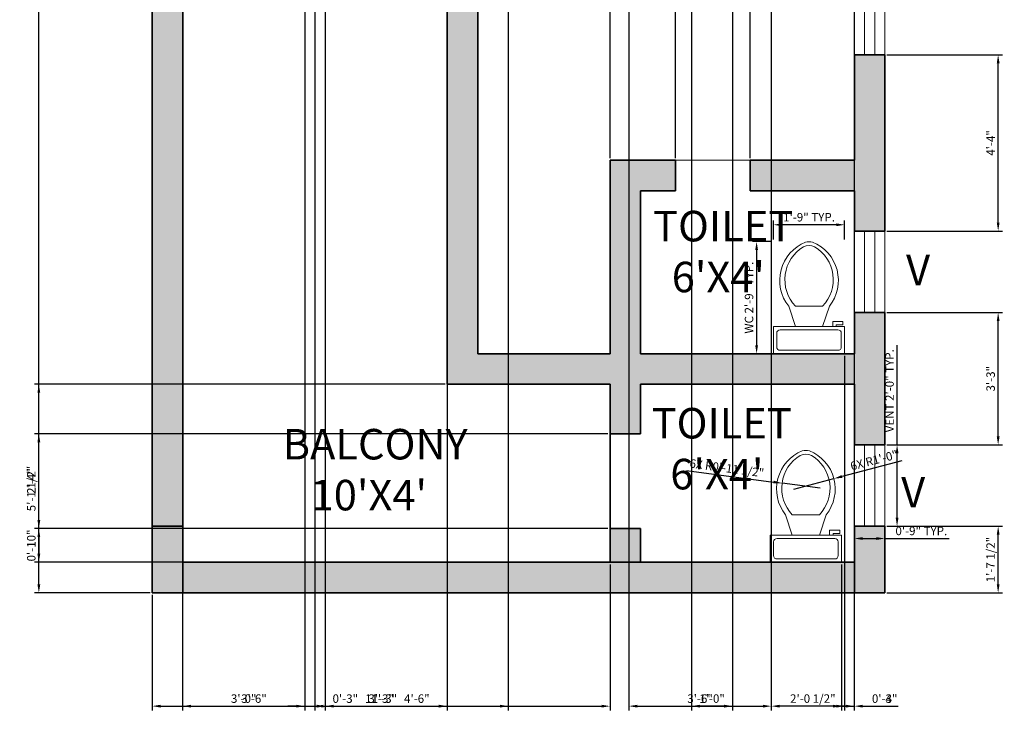
# Model space of a CAD drawing. Units: inches. Extents: x 4888 to 5178, y 5041 to 5743.
# Tile 1 of 3: x 4888 to 5178, y 5041 to 5245. Entities that reach past the tile are written whole.
import ezdxf

# ---------------------------------------------------------------- set-up
doc = ezdxf.new("R2010")
doc.units = ezdxf.units.IN
for name, color, linetype, lineweight in [('A-ANNO-DIMS', 2, 'Continuous', 18), ('A-ANNO-TEXT', 7, 'Continuous', 18), ('A-AREA-IDEN', 7, 'Continuous', 18), ('A-COLS', 7, 'Continuous', 35), ('A-DOOR', 4, 'Continuous', 18), ('A-FLOR-FIXT', 9, 'Continuous', 18), ('A-WALL', 7, 'Continuous', 35), ('A-WALL-PATT', 8, 'Continuous', 13)]:
    doc.layers.add(name, color=color, linetype=linetype, lineweight=lineweight)
doc.layers.add('A-COLS-PATT', color=18, linetype='Continuous', lineweight=13, true_color=0x000000)
doc.layers.add('A-GLAZ', color=31, linetype='Continuous', lineweight=18, true_color=0xfecc66)
doc.styles.get("Standard").update_dxf_attribs({"font": 'arial.ttf'})
doc.dimstyles.new('ISO-25', dxfattribs={"dimtxt": 2.5, "dimasz": 2.5, "dimexe": 1.25, "dimexo": 0.625, "dimtad": 1, "dimlunit": 3, "dimtxsty": 'Standard', "dimcen": 2.5, "dimadec": 0, "dimazin": 0, "dimtfac": 1, "dimtmove": 0, "dimatfit": 3, "dimfxl": 1, "dimarcsym": 0})

# ---------------------------------------------------------------- blocks, each defined once
blk = doc.blocks.new('Toilet - top')
for p, q in [((9.5, -6), (9.5, -2)), ((-10, -8.5), (-8, -8.5)), ((-10, -9.5), (-10, -8.5)), ((-8, -8.5), (-8, -8)), ((-7, -8), (-7, -9.5)), ((-4, -8), (-6, -14)), ((4, -8), (6, -14)), ((-7, -9.5), (-10, -9.5)), ((4, -14), (-4, -14))]:
    blk.add_line(p, q)
blk.add_lwpolyline([(10.5, -8), (10.5, 0), (-10.5, 0), (-10.5, -8)], close=True)
for points in [[(-9.5, -2), (-9.5, -6)], [(8.5, -1), (-8.5, -1)], [(-8.5, -7), (8.5, -7)]]:
    blk.add_lwpolyline(points)
for centre, radius, start, end in [((-8.62, -1.88), 0.884, 81.8699, 188.1301), ((8.62, -1.88), 0.884, 351.8699, 98.1301), ((-8.62, -6.12), 0.884, 171.8699, 278.1301), ((8.62, -6.12), 0.884, 261.8699, 8.1301), ((3.52, -21.58), 12.17, 141.4691, 247.9714), ((4.2, -21.82), 11.33, 136.3677, 238.9468), ((-3.52, -21.58), 12.17, 292.0284, 38.5307), ((-4.2, -21.82), 11.33, 301.053, 43.6321), ((0, -27.88), 4, 245.7318, 294.2682), ((0, -29), 4, 254.8605, 285.1395)]:
    blk.add_arc(centre, radius, start, end)
blk = doc.blocks.new('WIN-48IN')
for p, q in [((0, 9), (0, 0)), ((48, 9), (0, 9)), ((48, 0), (48, 9)), ((48, 6), (0, 6)), ((48, 3), (0, 3)), ((0, 0), (48, 0))]:
    blk.add_line(p, q)
blk = doc.blocks.new('VENT-24IN')
for p, q in [((0, 24), (0, 0)), ((9, 24), (0, 24)), ((3, 0), (3, 24)), ((6, 0), (6, 24)), ((9, 0), (9, 24)), ((0, 0), (9, 0))]:
    blk.add_line(p, q)
blk = doc.blocks.new('*D9')
at = {"layer": 'A-ANNO-DIMS', "color": 0, "lineweight": -2, "transparency": 16777216}
for p, q in [((5109.37, 5179.55), (5103.79, 5179.55)), ((5105.04, 5177.05), (5105.04, 5149.01)), ((5109.37, 5146.51), (5103.79, 5146.51))]:
    blk.add_line(p, q, dxfattribs=at)
at = {"layer": 'A-ANNO-DIMS', "color": 0, "transparency": 16777216}
for points in [[(5104.62, 5177.05), (5105.45, 5177.05), (5105.04, 5179.55)], [(5104.62, 5149.01), (5105.45, 5149.01), (5105.04, 5146.51)]]:
    blk.add_solid(points, dxfattribs=at)
at = {"layer": 'Defpoints', "color": 0, "transparency": 16777216}
for p in [(5109.99, 5179.55), (5105.04, 5146.51), (5109.99, 5146.51)]:
    blk.add_point(p, dxfattribs=at)
at = {"layer": 'A-ANNO-DIMS', "color": 0, "transparency": 16777216, "insert": (5103.12, 5163.03), "char_height": 2.5, "attachment_point": 5, "rotation": 90}
blk.add_mtext('WC 2\'-9" TYP.', dxfattribs=at)
blk = doc.blocks.new('*D10')
at = {"layer": 'A-ANNO-DIMS', "color": 0, "lineweight": -2, "transparency": 16777216}
for p, q in [((5109.99, 5180.18), (5109.99, 5185.76)), ((5128.49, 5184.51), (5112.49, 5184.51)), ((5130.99, 5180.18), (5130.99, 5185.76))]:
    blk.add_line(p, q, dxfattribs=at)
at = {"layer": 'A-ANNO-DIMS', "color": 0, "transparency": 16777216}
for points in [[(5112.49, 5184.93), (5112.49, 5184.09), (5109.99, 5184.51)], [(5128.49, 5184.93), (5128.49, 5184.09), (5130.99, 5184.51)]]:
    blk.add_solid(points, dxfattribs=at)
at = {"layer": 'Defpoints', "color": 0, "transparency": 16777216}
for p in [(5109.99, 5184.51), (5109.99, 5179.55), (5130.99, 5179.55)]:
    blk.add_point(p, dxfattribs=at)
at = {"layer": 'A-ANNO-DIMS', "color": 0, "transparency": 16777216, "insert": (5120.49, 5186.41), "char_height": 2.5, "attachment_point": 5}
blk.add_mtext('1\'-9" TYP.', dxfattribs=at)
blk = doc.blocks.new('*D11')
at = {"layer": 'A-ANNO-DIMS', "color": 0, "lineweight": -2, "transparency": 16777216}
for p, q in [((5146.44, 5119.63), (5146.44, 5149.03)), ((5143.47, 5119.63), (5147.69, 5119.63)), ((5146.44, 5098.13), (5146.44, 5117.13)), ((5143.47, 5095.63), (5147.69, 5095.63))]:
    blk.add_line(p, q, dxfattribs=at)
at = {"layer": 'A-ANNO-DIMS', "color": 0, "transparency": 16777216}
for points in [[(5146.03, 5117.13), (5146.86, 5117.13), (5146.44, 5119.63)], [(5146.03, 5098.13), (5146.86, 5098.13), (5146.44, 5095.63)]]:
    blk.add_solid(points, dxfattribs=at)
at = {"layer": 'Defpoints', "color": 0, "transparency": 16777216}
for p in [(5142.84, 5119.63), (5146.44, 5119.63), (5142.84, 5095.63)]:
    blk.add_point(p, dxfattribs=at)
at = {"layer": 'A-ANNO-DIMS', "color": 0, "transparency": 16777216, "insert": (5144.54, 5135.58), "char_height": 2.5, "attachment_point": 5, "rotation": 90}
blk.add_mtext('VENT 2\'-0" TYP.', dxfattribs=at)
blk = doc.blocks.new('*D12')
at = {"layer": 'A-ANNO-DIMS', "color": 0, "lineweight": -2, "transparency": 16777216}
for p, q in [((5133.84, 5095), (5133.84, 5090.78)), ((5142.84, 5095), (5142.84, 5090.78)), ((5136.34, 5092.03), (5140.34, 5092.03)), ((5142.84, 5092.03), (5161.83, 5092.03))]:
    blk.add_line(p, q, dxfattribs=at)
at = {"layer": 'A-ANNO-DIMS', "color": 0, "transparency": 16777216}
for points in [[(5136.34, 5092.44), (5136.34, 5091.61), (5133.84, 5092.03)], [(5140.34, 5092.44), (5140.34, 5091.61), (5142.84, 5092.03)]]:
    blk.add_solid(points, dxfattribs=at)
at = {"layer": 'Defpoints', "color": 0, "transparency": 16777216}
for p in [(5133.84, 5095.63), (5142.84, 5095.63), (5142.84, 5092.03)]:
    blk.add_point(p, dxfattribs=at)
at = {"layer": 'A-ANNO-DIMS', "color": 0, "transparency": 16777216, "insert": (5153.59, 5093.93), "char_height": 2.5, "attachment_point": 5}
blk.add_mtext('0\'-9" TYP.', dxfattribs=at)
blk = doc.blocks.new('*D17')
at = {"layer": 'A-ANNO-DIMS', "color": 0, "lineweight": -2, "transparency": 16777216}
for p, q in [((4926.22, 5685.01), (4892.19, 5685.01)), ((4893.44, 5078.51), (4893.44, 5682.51)), ((4926.22, 5076.01), (4892.19, 5076.01))]:
    blk.add_line(p, q, dxfattribs=at)
at = {"layer": 'A-ANNO-DIMS', "color": 0, "transparency": 16777216}
for points in [[(4893.03, 5682.51), (4893.86, 5682.51), (4893.44, 5685.01)], [(4893.03, 5078.51), (4893.86, 5078.51), (4893.44, 5076.01)]]:
    blk.add_solid(points, dxfattribs=at)
at = {"layer": 'Defpoints', "color": 0, "transparency": 16777216}
for p in [(4893.44, 5685.01), (4926.84, 5685.01), (4926.84, 5076.01)]:
    blk.add_point(p, dxfattribs=at)
at = {"layer": 'A-ANNO-DIMS', "color": 0, "transparency": 16777216, "insert": (4891.54, 5380.51), "char_height": 2.5, "attachment_point": 5, "rotation": 90}
blk.add_mtext('50\'-9"', dxfattribs=at)
blk = doc.blocks.new('*D21')
at = {"layer": 'A-ANNO-DIMS', "color": 0, "lineweight": -2, "transparency": 16777216}
for p, q in [((5143.47, 5095.63), (5177.49, 5095.63)), ((5176.24, 5078.51), (5176.24, 5093.13)), ((5143.47, 5076.01), (5177.49, 5076.01))]:
    blk.add_line(p, q, dxfattribs=at)
at = {"layer": 'A-ANNO-DIMS', "color": 0, "transparency": 16777216}
for points in [[(5175.83, 5093.13), (5176.66, 5093.13), (5176.24, 5095.63)], [(5175.83, 5078.51), (5176.66, 5078.51), (5176.24, 5076.01)]]:
    blk.add_solid(points, dxfattribs=at)
at = {"layer": 'Defpoints', "color": 0, "transparency": 16777216}
for p in [(5142.84, 5095.63), (5176.24, 5095.63), (5142.84, 5076.01)]:
    blk.add_point(p, dxfattribs=at)
at = {"layer": 'A-ANNO-DIMS', "color": 0, "transparency": 16777216, "insert": (5174.33, 5085.82), "char_height": 2.5, "attachment_point": 5, "rotation": 90}
blk.add_mtext('1\'-7 1/2"', dxfattribs=at)
blk = doc.blocks.new('*D22')
at = {"layer": 'A-ANNO-DIMS', "color": 0, "lineweight": -2, "transparency": 16777216}
for p, q in [((5143.47, 5158.64), (5177.49, 5158.64)), ((5176.24, 5122.13), (5176.24, 5156.14)), ((5143.47, 5119.63), (5177.49, 5119.63))]:
    blk.add_line(p, q, dxfattribs=at)
at = {"layer": 'A-ANNO-DIMS', "color": 0, "transparency": 16777216}
for points in [[(5175.83, 5156.14), (5176.66, 5156.14), (5176.24, 5158.64)], [(5175.83, 5122.13), (5176.66, 5122.13), (5176.24, 5119.63)]]:
    blk.add_solid(points, dxfattribs=at)
at = {"layer": 'Defpoints', "color": 0, "transparency": 16777216}
for p in [(5142.84, 5158.64), (5176.24, 5158.64), (5142.84, 5119.63)]:
    blk.add_point(p, dxfattribs=at)
at = {"layer": 'A-ANNO-DIMS', "color": 0, "transparency": 16777216, "insert": (5174.34, 5139.13), "char_height": 2.5, "attachment_point": 5, "rotation": 90}
blk.add_mtext('3\'-3"', dxfattribs=at)
blk = doc.blocks.new('*D23')
at = {"layer": 'A-ANNO-DIMS', "color": 0, "lineweight": -2, "transparency": 16777216}
for p, q in [((5143.47, 5234.61), (5177.49, 5234.61)), ((5176.24, 5185.14), (5176.24, 5232.11)), ((5143.47, 5182.64), (5177.49, 5182.64))]:
    blk.add_line(p, q, dxfattribs=at)
at = {"layer": 'A-ANNO-DIMS', "color": 0, "transparency": 16777216}
for points in [[(5175.83, 5232.11), (5176.66, 5232.11), (5176.24, 5234.61)], [(5175.83, 5185.14), (5176.66, 5185.14), (5176.24, 5182.64)]]:
    blk.add_solid(points, dxfattribs=at)
at = {"layer": 'Defpoints', "color": 0, "transparency": 16777216}
for p in [(5142.84, 5234.61), (5176.24, 5234.61), (5142.84, 5182.64)]:
    blk.add_point(p, dxfattribs=at)
at = {"layer": 'A-ANNO-DIMS', "color": 0, "transparency": 16777216, "insert": (5174.37, 5208.63), "char_height": 2.5, "attachment_point": 5, "rotation": 90}
blk.add_mtext('4\'-4"', dxfattribs=at)
blk = doc.blocks.new('*D28')
at = {"layer": 'A-ANNO-DIMS', "color": 0, "lineweight": -2, "transparency": 16777216}
for p, q in [((4935.84, 5330.38), (4935.84, 5041.36)), ((4971.84, 5330.38), (4971.84, 5041.36)), ((4938.34, 5042.61), (4969.34, 5042.61))]:
    blk.add_line(p, q, dxfattribs=at)
at = {"layer": 'A-ANNO-DIMS', "color": 0, "transparency": 16777216}
for points in [[(4938.34, 5043.02), (4938.34, 5042.19), (4935.84, 5042.61)], [(4969.34, 5043.02), (4969.34, 5042.19), (4971.84, 5042.61)]]:
    blk.add_solid(points, dxfattribs=at)
at = {"layer": 'Defpoints', "color": 0, "transparency": 16777216}
for p in [(4935.84, 5331.01), (4971.84, 5331.01), (4971.84, 5042.61)]:
    blk.add_point(p, dxfattribs=at)
at = {"layer": 'A-ANNO-DIMS', "color": 0, "transparency": 16777216, "insert": (4953.84, 5044.51), "char_height": 2.5, "attachment_point": 5}
blk.add_mtext('3\'-0"', dxfattribs=at)
blk = doc.blocks.new('*D29')
at = {"layer": 'A-ANNO-DIMS', "color": 0, "lineweight": -2, "transparency": 16777216}
for p, q in [((5067.37, 5322.88), (5067.37, 5041.36)), ((5109.37, 5322.88), (5109.37, 5041.36)), ((5069.87, 5042.61), (5106.87, 5042.61))]:
    blk.add_line(p, q, dxfattribs=at)
at = {"layer": 'A-ANNO-DIMS', "color": 0, "transparency": 16777216}
for points in [[(5069.87, 5043.02), (5069.87, 5042.19), (5067.37, 5042.61)], [(5106.87, 5043.02), (5106.87, 5042.19), (5109.37, 5042.61)]]:
    blk.add_solid(points, dxfattribs=at)
at = {"layer": 'Defpoints', "color": 0, "transparency": 16777216}
for p in [(5067.37, 5323.51), (5109.37, 5323.51), (5109.37, 5042.61)]:
    blk.add_point(p, dxfattribs=at)
at = {"layer": 'A-ANNO-DIMS', "color": 0, "transparency": 16777216, "insert": (5088.37, 5044.51), "char_height": 2.5, "attachment_point": 5}
blk.add_mtext('3\'-6"', dxfattribs=at)
blk = doc.blocks.new('*D30')
at = {"layer": 'A-ANNO-DIMS', "color": 0, "lineweight": -2, "transparency": 16777216}
for p, q in [((5109.37, 5322.88), (5109.37, 5041.36)), ((5133.84, 5322.88), (5133.84, 5041.36)), ((5131.34, 5042.61), (5111.87, 5042.61))]:
    blk.add_line(p, q, dxfattribs=at)
at = {"layer": 'A-ANNO-DIMS', "color": 0, "transparency": 16777216}
for points in [[(5111.87, 5043.02), (5111.87, 5042.19), (5109.37, 5042.61)], [(5131.34, 5043.02), (5131.34, 5042.19), (5133.84, 5042.61)]]:
    blk.add_solid(points, dxfattribs=at)
at = {"layer": 'Defpoints', "color": 0, "transparency": 16777216}
for p in [(5109.37, 5323.51), (5133.84, 5323.51), (5109.37, 5042.61)]:
    blk.add_point(p, dxfattribs=at)
at = {"layer": 'A-ANNO-DIMS', "color": 0, "transparency": 16777216, "insert": (5121.61, 5044.52), "char_height": 2.5, "attachment_point": 5}
blk.add_mtext('2\'-0 1/2"', dxfattribs=at)
blk = doc.blocks.new('*D32')
at = {"layer": 'A-ANNO-DIMS', "color": 0, "lineweight": -2, "transparency": 16777216}
for p, q in [((4977.89, 5550.88), (4977.89, 5041.36)), ((5031.84, 5550.88), (5031.84, 5041.36)), ((4980.39, 5042.61), (5029.34, 5042.61))]:
    blk.add_line(p, q, dxfattribs=at)
at = {"layer": 'A-ANNO-DIMS', "color": 0, "transparency": 16777216}
for points in [[(4980.39, 5043.02), (4980.39, 5042.19), (4977.89, 5042.61)], [(5029.34, 5043.02), (5029.34, 5042.19), (5031.84, 5042.61)]]:
    blk.add_solid(points, dxfattribs=at)
at = {"layer": 'Defpoints', "color": 0, "transparency": 16777216}
for p in [(4977.89, 5551.51), (5031.84, 5551.51), (5031.84, 5042.61)]:
    blk.add_point(p, dxfattribs=at)
at = {"layer": 'A-ANNO-DIMS', "color": 0, "transparency": 16777216, "insert": (5004.87, 5044.51), "char_height": 2.5, "attachment_point": 5}
blk.add_mtext('4\'-6"', dxfattribs=at)
blk = doc.blocks.new('*D36')
at = {"layer": 'A-ANNO-DIMS', "color": 0, "lineweight": -2, "transparency": 16777216}
for p, q in [((5081.08, 5204.13), (5081.08, 5719.66)), ((5083.58, 5718.41), (5100.61, 5718.41)), ((5103.11, 5204.13), (5103.11, 5719.66))]:
    blk.add_line(p, q, dxfattribs=at)
at = {"layer": 'A-ANNO-DIMS', "color": 0, "transparency": 16777216}
for points in [[(5083.58, 5718.82), (5083.58, 5717.99), (5081.08, 5718.41)], [(5100.61, 5718.82), (5100.61, 5717.99), (5103.11, 5718.41)]]:
    blk.add_solid(points, dxfattribs=at)
at = {"layer": 'Defpoints', "color": 0, "transparency": 16777216}
for p in [(5103.11, 5718.41), (5081.08, 5203.51), (5103.11, 5203.51)]:
    blk.add_point(p, dxfattribs=at)
at = {"layer": 'A-ANNO-DIMS', "color": 0, "transparency": 16777216, "insert": (5092.09, 5720.31), "char_height": 2.5, "attachment_point": 5}
blk.add_mtext('1\'-10"', dxfattribs=at)
blk = doc.blocks.new('*D37')
at = {"layer": 'A-ANNO-DIMS', "color": 0, "lineweight": -2, "transparency": 16777216}
for p, q in [((5061.22, 5122.91), (4892.19, 5122.91)), ((4893.44, 5097.46), (4893.44, 5120.41)), ((5061.22, 5094.96), (4892.19, 5094.96))]:
    blk.add_line(p, q, dxfattribs=at)
at = {"layer": 'A-ANNO-DIMS', "color": 0, "transparency": 16777216}
for points in [[(4893.03, 5120.41), (4893.86, 5120.41), (4893.44, 5122.91)], [(4893.03, 5097.46), (4893.86, 5097.46), (4893.44, 5094.96)]]:
    blk.add_solid(points, dxfattribs=at)
at = {"layer": 'Defpoints', "color": 0, "transparency": 16777216}
for p in [(4893.44, 5122.91), (5061.84, 5122.91), (5061.84, 5094.96)]:
    blk.add_point(p, dxfattribs=at)
at = {"layer": 'A-ANNO-DIMS', "color": 0, "transparency": 16777216, "insert": (4891.56, 5108.94), "char_height": 2.5, "attachment_point": 5, "rotation": 90}
blk.add_mtext('2\'-4"', dxfattribs=at)
blk = doc.blocks.new('*D39')
at = {"layer": 'A-ANNO-DIMS', "color": 0, "lineweight": -2, "transparency": 16777216}
for p, q in [((4935.84, 5555.38), (4935.84, 5041.36)), ((4977.89, 5555.38), (4977.89, 5041.36)), ((4938.34, 5042.61), (4975.39, 5042.61))]:
    blk.add_line(p, q, dxfattribs=at)
at = {"layer": 'A-ANNO-DIMS', "color": 0, "transparency": 16777216}
for points in [[(4938.34, 5043.02), (4938.34, 5042.19), (4935.84, 5042.61)], [(4975.39, 5043.02), (4975.39, 5042.19), (4977.89, 5042.61)]]:
    blk.add_solid(points, dxfattribs=at)
at = {"layer": 'Defpoints', "color": 0, "transparency": 16777216}
for p in [(4935.84, 5556.01), (4977.89, 5556.01), (4977.89, 5042.61)]:
    blk.add_point(p, dxfattribs=at)
at = {"layer": 'A-ANNO-DIMS', "color": 0, "transparency": 16777216, "insert": (4956.87, 5044.51), "char_height": 2.5, "attachment_point": 5}
blk.add_mtext('3\'-6"', dxfattribs=at)
blk = doc.blocks.new('*D40')
at = {"layer": 'A-ANNO-DIMS', "color": 0, "lineweight": -2, "transparency": 16777216}
for p, q in [((5061.84, 5204.13), (5061.84, 5719.66)), ((5064.34, 5718.41), (5078.58, 5718.41)), ((5081.08, 5204.13), (5081.08, 5719.66))]:
    blk.add_line(p, q, dxfattribs=at)
at = {"layer": 'A-ANNO-DIMS', "color": 0, "transparency": 16777216}
for points in [[(5064.34, 5718.82), (5064.34, 5717.99), (5061.84, 5718.41)], [(5078.58, 5718.82), (5078.58, 5717.99), (5081.08, 5718.41)]]:
    blk.add_solid(points, dxfattribs=at)
at = {"layer": 'Defpoints', "color": 0, "transparency": 16777216}
for p in [(5081.08, 5718.41), (5061.84, 5203.51), (5081.08, 5203.51)]:
    blk.add_point(p, dxfattribs=at)
at = {"layer": 'A-ANNO-DIMS', "color": 0, "transparency": 16777216, "insert": (5071.46, 5720.29), "char_height": 2.5, "attachment_point": 5}
blk.add_mtext('1\'-7"', dxfattribs=at)
blk = doc.blocks.new('*D41')
at = {"layer": 'A-ANNO-DIMS', "color": 0, "lineweight": -2, "transparency": 16777216}
for p, q in [((5061.22, 5094.96), (4892.19, 5094.96)), ((4893.44, 5092.46), (4893.44, 5087.51)), ((5061.22, 5085.01), (4892.19, 5085.01))]:
    blk.add_line(p, q, dxfattribs=at)
at = {"layer": 'A-ANNO-DIMS', "color": 0, "transparency": 16777216}
for points in [[(4893.03, 5092.46), (4893.86, 5092.46), (4893.44, 5094.96)], [(4893.03, 5087.51), (4893.86, 5087.51), (4893.44, 5085.01)]]:
    blk.add_solid(points, dxfattribs=at)
at = {"layer": 'Defpoints', "color": 0, "transparency": 16777216}
for p in [(5061.84, 5094.96), (4893.44, 5085.01), (5061.84, 5085.01)]:
    blk.add_point(p, dxfattribs=at)
at = {"layer": 'A-ANNO-DIMS', "color": 0, "transparency": 16777216, "insert": (4891.54, 5089.98), "char_height": 2.5, "attachment_point": 5, "rotation": 90}
blk.add_mtext('0\'-10"', dxfattribs=at)
blk = doc.blocks.new('*D45')
at = {"layer": 'A-ANNO-DIMS', "color": 0, "lineweight": -2, "transparency": 16777216}
for p, q in [((5130.99, 5145.88), (5130.99, 5041.36)), ((5133.84, 5145.88), (5133.84, 5041.36)), ((5128.49, 5042.61), (5125.99, 5042.61)), ((5130.99, 5042.61), (5133.84, 5042.61)), ((5136.34, 5042.61), (5146.74, 5042.61))]:
    blk.add_line(p, q, dxfattribs=at)
at = {"layer": 'A-ANNO-DIMS', "color": 0, "transparency": 16777216}
for points in [[(5128.49, 5043.02), (5128.49, 5042.19), (5130.99, 5042.61)], [(5136.34, 5043.02), (5136.34, 5042.19), (5133.84, 5042.61)]]:
    blk.add_solid(points, dxfattribs=at)
at = {"layer": 'Defpoints', "color": 0, "transparency": 16777216}
for p in [(5130.99, 5146.51), (5133.84, 5146.51), (5133.84, 5042.61)]:
    blk.add_point(p, dxfattribs=at)
at = {"layer": 'A-ANNO-DIMS', "color": 0, "transparency": 16777216, "insert": (5142.79, 5044.51), "char_height": 2.5, "attachment_point": 5}
blk.add_mtext('0\'-3"', dxfattribs=at)
blk = doc.blocks.new('*D46')
at = {"layer": 'A-ANNO-DIMS', "color": 0, "lineweight": -2, "transparency": 16777216}
for p, q in [((5130.06, 5084.38), (5130.06, 5041.36)), ((5133.84, 5084.38), (5133.84, 5041.36)), ((5127.56, 5042.61), (5125.06, 5042.61)), ((5130.06, 5042.61), (5133.84, 5042.61)), ((5136.34, 5042.61), (5146.74, 5042.61))]:
    blk.add_line(p, q, dxfattribs=at)
at = {"layer": 'A-ANNO-DIMS', "color": 0, "transparency": 16777216}
for points in [[(5127.56, 5043.02), (5127.56, 5042.19), (5130.06, 5042.61)], [(5136.34, 5043.02), (5136.34, 5042.19), (5133.84, 5042.61)]]:
    blk.add_solid(points, dxfattribs=at)
at = {"layer": 'Defpoints', "color": 0, "transparency": 16777216}
for p in [(5130.06, 5085.01), (5133.84, 5085.01), (5133.84, 5042.61)]:
    blk.add_point(p, dxfattribs=at)
at = {"layer": 'A-ANNO-DIMS', "color": 0, "transparency": 16777216, "insert": (5142.79, 5044.51), "char_height": 2.5, "attachment_point": 5}
blk.add_mtext('0\'-4"', dxfattribs=at)
blk = doc.blocks.new('*D47')
at = {"layer": 'A-ANNO-DIMS', "color": 0, "lineweight": -2, "transparency": 16777216}
for p, q in [((5061.84, 5084.38), (5061.84, 5041.36)), ((4926.84, 5075.38), (4926.84, 5041.36)), ((4929.34, 5042.61), (5059.34, 5042.61))]:
    blk.add_line(p, q, dxfattribs=at)
at = {"layer": 'A-ANNO-DIMS', "color": 0, "transparency": 16777216}
for points in [[(4929.34, 5043.02), (4929.34, 5042.19), (4926.84, 5042.61)], [(5059.34, 5043.02), (5059.34, 5042.19), (5061.84, 5042.61)]]:
    blk.add_solid(points, dxfattribs=at)
at = {"layer": 'Defpoints', "color": 0, "transparency": 16777216}
for p in [(5061.84, 5085.01), (4926.84, 5076.01), (5061.84, 5042.61)]:
    blk.add_point(p, dxfattribs=at)
at = {"layer": 'A-ANNO-DIMS', "color": 0, "transparency": 16777216, "insert": (4994.34, 5044.51), "char_height": 2.5, "attachment_point": 5}
blk.add_mtext('11\'-3"', dxfattribs=at)
blk = doc.blocks.new('*D48')
at = {"layer": 'A-ANNO-DIMS', "color": 0, "lineweight": -2, "transparency": 16777216}
for p, q in [((5013.22, 5137.51), (4892.19, 5137.51)), ((4893.44, 5078.51), (4893.44, 5135.01)), ((4926.22, 5076.01), (4892.19, 5076.01))]:
    blk.add_line(p, q, dxfattribs=at)
at = {"layer": 'A-ANNO-DIMS', "color": 0, "transparency": 16777216}
for points in [[(4893.03, 5135.01), (4893.86, 5135.01), (4893.44, 5137.51)], [(4893.03, 5078.51), (4893.86, 5078.51), (4893.44, 5076.01)]]:
    blk.add_solid(points, dxfattribs=at)
at = {"layer": 'Defpoints', "color": 0, "transparency": 16777216}
for p in [(4893.44, 5137.51), (5013.84, 5137.51), (4926.84, 5076.01)]:
    blk.add_point(p, dxfattribs=at)
at = {"layer": 'A-ANNO-DIMS', "color": 0, "transparency": 16777216, "insert": (4891.53, 5106.76), "char_height": 2.5, "attachment_point": 5, "rotation": 90}
blk.add_mtext('5\'-1 1/2"', dxfattribs=at)
blk = doc.blocks.new('*D50')
at = {"layer": 'A-ANNO-DIMS', "color": 0, "lineweight": -2, "transparency": 16777216}
for p, q in [((5085.84, 5466.88), (5085.84, 5041.36)), ((5097.97, 5466.88), (5097.97, 5041.36)), ((5095.47, 5042.61), (5088.34, 5042.61))]:
    blk.add_line(p, q, dxfattribs=at)
at = {"layer": 'A-ANNO-DIMS', "color": 0, "transparency": 16777216}
for points in [[(5088.34, 5043.02), (5088.34, 5042.19), (5085.84, 5042.61)], [(5095.47, 5043.02), (5095.47, 5042.19), (5097.97, 5042.61)]]:
    blk.add_solid(points, dxfattribs=at)
at = {"layer": 'Defpoints', "color": 0, "transparency": 16777216}
for p in [(5085.84, 5467.51), (5097.97, 5467.51), (5085.84, 5042.61)]:
    blk.add_point(p, dxfattribs=at)
at = {"layer": 'A-ANNO-DIMS', "color": 0, "transparency": 16777216, "insert": (5091.91, 5044.51), "char_height": 2.5, "attachment_point": 5}
blk.add_mtext('1\'-0"', dxfattribs=at)
blk = doc.blocks.new('*D51')
at = {"layer": 'A-ANNO-DIMS', "color": 0, "lineweight": -2, "transparency": 16777216}
for p, q in [((4971.84, 5330.38), (4971.84, 5041.36)), ((4974.84, 5330.38), (4974.84, 5041.36)), ((4969.34, 5042.61), (4966.84, 5042.61)), ((4971.84, 5042.61), (4974.84, 5042.61)), ((4977.34, 5042.61), (4987.74, 5042.61))]:
    blk.add_line(p, q, dxfattribs=at)
at = {"layer": 'A-ANNO-DIMS', "color": 0, "transparency": 16777216}
for points in [[(4969.34, 5043.02), (4969.34, 5042.19), (4971.84, 5042.61)], [(4977.34, 5043.02), (4977.34, 5042.19), (4974.84, 5042.61)]]:
    blk.add_solid(points, dxfattribs=at)
at = {"layer": 'Defpoints', "color": 0, "transparency": 16777216}
for p in [(4971.84, 5331.01), (4974.84, 5331.01), (4974.84, 5042.61)]:
    blk.add_point(p, dxfattribs=at)
at = {"layer": 'A-ANNO-DIMS', "color": 0, "transparency": 16777216, "insert": (4983.79, 5044.51), "char_height": 2.5, "attachment_point": 5}
blk.add_mtext('0\'-3"', dxfattribs=at)
blk = doc.blocks.new('*D52')
at = {"layer": 'A-ANNO-DIMS', "color": 0, "lineweight": -2, "transparency": 16777216}
for p, q in [((4974.84, 5342.38), (4974.84, 5041.36)), ((5013.84, 5342.38), (5013.84, 5041.36)), ((4977.34, 5042.61), (5011.34, 5042.61))]:
    blk.add_line(p, q, dxfattribs=at)
at = {"layer": 'A-ANNO-DIMS', "color": 0, "transparency": 16777216}
for points in [[(4977.34, 5043.02), (4977.34, 5042.19), (4974.84, 5042.61)], [(5011.34, 5043.02), (5011.34, 5042.19), (5013.84, 5042.61)]]:
    blk.add_solid(points, dxfattribs=at)
at = {"layer": 'Defpoints', "color": 0, "transparency": 16777216}
for p in [(4974.84, 5343.01), (5013.84, 5343.01), (5013.84, 5042.61)]:
    blk.add_point(p, dxfattribs=at)
at = {"layer": 'A-ANNO-DIMS', "color": 0, "transparency": 16777216, "insert": (4994.34, 5044.51), "char_height": 2.5, "attachment_point": 5}
blk.add_mtext('3\'-3"', dxfattribs=at)
blk = doc.blocks.new('*D55')
at = {"layer": 'A-ANNO-DIMS', "color": 0, "lineweight": -2, "transparency": 16777216}
for p, q in [((5147.8, 5114.93), (5130.22, 5110.31)), ((5116.04, 5106.59), (5127.81, 5109.68))]:
    blk.add_line(p, q, dxfattribs=at)
at = {"layer": 'A-ANNO-DIMS', "color": 0, "transparency": 16777216}
blk.add_solid([(5130.12, 5110.72), (5130.33, 5109.91), (5127.81, 5109.68)], dxfattribs=at)
at = {"layer": 'Defpoints', "color": 0, "transparency": 16777216}
for p in [(5127.81, 5109.68), (5116.04, 5106.59)]:
    blk.add_point(p, dxfattribs=at)
at = {"layer": 'A-ANNO-DIMS', "color": 0, "transparency": 16777216, "insert": (5139.74, 5114.78), "char_height": 2.5, "attachment_point": 5, "rotation": 14.7224}
blk.add_mtext('6X R1\'-0"', dxfattribs=at)
blk = doc.blocks.new('*D56')
at = {"layer": 'A-ANNO-DIMS', "color": 0, "lineweight": -2, "transparency": 16777216}
for p, q in [((5084.34, 5112.12), (5110.05, 5108.67)), ((5123.76, 5106.82), (5112.53, 5108.33))]:
    blk.add_line(p, q, dxfattribs=at)
at = {"layer": 'A-ANNO-DIMS', "color": 0, "transparency": 16777216}
blk.add_solid([(5110.11, 5109.08), (5109.99, 5108.25), (5112.53, 5108.33)], dxfattribs=at)
at = {"layer": 'Defpoints', "color": 0, "transparency": 16777216}
for p in [(5112.53, 5108.33), (5123.76, 5106.82)]:
    blk.add_point(p, dxfattribs=at)
at = {"layer": 'A-ANNO-DIMS', "color": 0, "transparency": 16777216, "insert": (5096.21, 5112.46), "char_height": 2.5, "attachment_point": 5, "rotation": 352.3419}
blk.add_mtext('6X R0\'-11 1/2"', dxfattribs=at)

msp = doc.modelspace()

# ---------------------------------------------------------------- hatches: boundary and pattern name
at = {"layer": 'A-COLS-PATT'}
h = msp.add_hatch(color=256, dxfattribs=at)
h.dxf.hatch_style = 1
h.paths.add_polyline_path([(4935.844, 5685.006), (4926.844, 5685.006), (4926.844, 5669.086), (4935.844, 5669.086)])
h.paths.add_polyline_path([(5142.844, 5685.006), (5133.844, 5685.006), (5133.844, 5669.086), (5142.844, 5669.086)])
h.paths.add_polyline_path([(4935.844, 5467.506), (4926.844, 5467.506), (4926.844, 5455.506), (4926.844, 5446.68), (4935.844, 5446.68)])
h.paths.add_polyline_path([(5142.844, 5467.506), (5133.844, 5467.506), (5133.844, 5446.68), (5142.844, 5446.68)])
h.paths.add_polyline_path([(4935.844, 5340.228), (4926.844, 5340.228), (4926.844, 5313.351), (4935.844, 5313.351)])
h.paths.add_polyline_path([(4935.844, 5095.626), (4926.844, 5095.626), (4926.844, 5076.006), (4935.844, 5076.006)])
h.paths.add_polyline_path([(5142.844, 5095.626), (5133.844, 5095.626), (5133.844, 5076.006), (5142.844, 5076.006)])
at = {"layer": 'A-WALL-PATT'}
h = msp.add_hatch(color=256, dxfattribs=at)
h.dxf.hatch_style = 1
h.paths.add_polyline_path([(5050.684, 5685.006), (4935.844, 5685.006), (4935.844, 5676.006), (5031.844, 5676.006), (5031.844, 5551.506), (5039.344, 5551.506), (5039.344, 5556.006), (5036.344, 5556.006), (5036.344, 5676.006), (5050.684, 5676.006)])
h.paths.add_polyline_path([(4935.844, 5669.086), (4926.844, 5669.086), (4926.844, 5610.401), (4935.844, 5610.401)])
h.paths.add_polyline_path([(5133.844, 5685.006), (5098.684, 5685.006), (5098.684, 5676.006), (5133.844, 5676.006)])
h.paths.add_polyline_path([(5142.844, 5669.086), (5133.844, 5669.086), (5133.844, 5556.006), (5109.899, 5556.006), (5109.899, 5551.506), (5133.844, 5551.506), (5133.844, 5524.266), (5142.844, 5524.266)])
h.paths.add_polyline_path([(4977.891, 5556.006), (4935.844, 5556.006), (4935.844, 5562.401), (4926.844, 5562.401), (4926.844, 5528.1), (4935.844, 5528.1), (4935.844, 5551.506), (4977.891, 5551.506)])
h.paths.add_polyline_path([(4935.844, 5480.1), (4926.844, 5480.1), (4926.844, 5467.506), (4935.844, 5467.506)])
h.paths.add_polyline_path([(5022.844, 5467.506), (4935.844, 5467.506), (4935.844, 5463.006), (5013.844, 5463.006), (5013.844, 5388.655), (5022.844, 5388.655)])
h.paths.add_polyline_path([(5133.844, 5467.506), (5085.844, 5467.506), (5085.844, 5551.506), (5091.899, 5551.506), (5091.899, 5556.006), (5081.344, 5556.006), (5081.344, 5463.006), (5133.844, 5463.006)])
h.paths.add_polyline_path([(5142.844, 5500.266), (5133.844, 5500.266), (5133.844, 5467.506), (5142.844, 5467.506)])
h.paths.add_polyline_path([(5142.844, 5446.68), (5133.844, 5446.68), (5133.844, 5420.006), (5142.844, 5420.006)])
h.paths.add_polyline_path([(5022.844, 5323.506), (5067.366, 5323.506), (5067.366, 5328.006), (5022.844, 5328.006), (5022.844, 5340.655), (5013.844, 5340.655), (5013.844, 5137.506), (5061.844, 5137.506), (5061.844, 5122.915), (5070.844, 5122.915), (5070.844, 5137.506), (5133.844, 5137.506), (5133.844, 5119.626), (5142.844, 5119.626), (5142.844, 5158.641), (5133.844, 5158.641), (5133.844, 5146.506), (5070.844, 5146.506), (5070.844, 5194.506), (5081.079, 5194.506), (5081.079, 5203.506), (5061.844, 5203.506), (5061.844, 5146.506), (5022.844, 5146.506)])
h.paths.add_polyline_path([(4935.844, 5313.351), (4926.844, 5313.351), (4926.844, 5095.626), (4935.844, 5095.626)])
h.paths.add_polyline_path([(4935.844, 5446.68), (4926.844, 5446.68), (4926.844, 5340.228), (4935.844, 5340.228)])
h.paths.add_polyline_path([(5142.844, 5372.006), (5133.844, 5372.006), (5133.844, 5340.228), (5142.844, 5340.228)])
h.paths.add_polyline_path([(5133.844, 5328.006), (5109.366, 5328.006), (5109.366, 5323.506), (5133.844, 5323.506)], flags=17)
h.paths.add_polyline_path([(5142.844, 5313.351), (5133.844, 5313.351), (5133.844, 5282.61), (5142.844, 5282.61)], flags=17)
h.paths.add_polyline_path([(5142.844, 5234.61), (5133.844, 5234.61), (5133.844, 5203.506), (5103.109, 5203.506), (5103.109, 5194.506), (5133.844, 5194.506), (5133.844, 5182.641), (5142.844, 5182.641)], flags=17)
h.paths.add_polyline_path([(5133.844, 5085.006), (4935.844, 5085.006), (4935.844, 5076.006), (5133.844, 5076.006)])
h.paths.add_polyline_path([(5070.844, 5094.96), (5061.844, 5094.96), (5061.844, 5085.006), (5070.844, 5085.006)])

# ---------------------------------------------------------------- linework, layer by layer
at = {"layer": 'A-COLS'}
msp.add_line((4935.844, 5095.626), (4926.844, 5095.626), dxfattribs=at)
at = {"layer": 'A-DOOR'}
msp.add_line((5081.079, 5203.506), (5103.109, 5203.506), dxfattribs=at)
at = {"layer": 'A-WALL'}
for p, q in [((4926.844, 5076.006), (4926.844, 5480.1)), ((4935.844, 5076.006), (4935.844, 5467.506)), ((5013.844, 5463.006), (5013.844, 5137.506)), ((5022.844, 5323.506), (5022.844, 5146.506)), ((5133.844, 5234.61), (5142.844, 5234.61)), ((5133.844, 5234.61), (5133.844, 5203.506)), ((5142.844, 5234.61), (5142.844, 5182.641)), ((5061.844, 5203.506), (5081.079, 5203.506)), ((5061.844, 5203.506), (5061.844, 5146.506)), ((5081.079, 5203.506), (5081.079, 5194.506)), ((5103.109, 5203.506), (5133.844, 5203.506)), ((5103.109, 5203.506), (5103.109, 5194.506)), ((5070.844, 5194.506), (5081.079, 5194.506)), ((5070.844, 5194.506), (5070.844, 5146.506)), ((5103.109, 5194.506), (5133.844, 5194.506)), ((5133.844, 5194.506), (5133.844, 5182.641)), ((5133.844, 5182.641), (5142.844, 5182.641)), ((5133.844, 5158.641), (5142.844, 5158.641)), ((5133.844, 5158.641), (5133.844, 5146.506)), ((5142.844, 5158.641), (5142.844, 5119.626)), ((5022.844, 5146.506), (5061.844, 5146.506)), ((5070.844, 5146.506), (5133.844, 5146.506)), ((5013.844, 5137.506), (5061.844, 5137.506)), ((5061.844, 5137.506), (5061.844, 5085.006)), ((5070.844, 5137.506), (5070.844, 5122.915)), ((5070.844, 5137.506), (5133.844, 5137.506)), ((5133.844, 5137.506), (5133.844, 5119.626)), ((5061.844, 5122.915), (5070.844, 5122.915)), ((5133.844, 5119.626), (5142.844, 5119.626)), ((5070.844, 5094.96), (5061.844, 5094.96)), ((5070.844, 5094.96), (5070.844, 5085.006)), ((5070.844, 5085.006), (5070.844, 5094.96)), ((5133.844, 5095.626), (5142.844, 5095.626)), ((5133.844, 5095.626), (5133.844, 5076.006)), ((5142.844, 5095.626), (5142.844, 5076.006)), ((5133.844, 5085.006), (4935.844, 5085.006)), ((5142.844, 5076.006), (4926.844, 5076.006))]:
    msp.add_line(p, q, dxfattribs=at)

# ---------------------------------------------------------------- block references
at = {"layer": 'A-FLOR-FIXT', "rotation": 180}
for p in [(5120.493, 5146.506), (5119.556, 5085.006)]:
    msp.add_blockref('Toilet - top', p, dxfattribs=at)
at = {"layer": 'A-GLAZ', "rotation": 90.00000000000003}
msp.add_blockref('WIN-48IN', (5142.844, 5234.61), dxfattribs=at)
at = {"layer": 'A-GLAZ'}
for p in [(5133.844, 5158.641), (5133.844, 5095.626)]:
    msp.add_blockref('VENT-24IN', p, dxfattribs=at)

# ---------------------------------------------------------------- texts
at = {"layer": 'A-ANNO-TEXT', "char_height": 9, "attachment_point": 1}
for insert in [(5149.096, 5175.677), (5149.096, 5175.677), (5147.653, 5110.178)]:
    msp.add_mtext_dynamic_manual_height_columns('V', width=76.41803, gutter_width=12.5, heights=[0], dxfattribs=dict(at, insert=insert))
at = {"layer": 'A-AREA-IDEN', "char_height": 9, "attachment_point": 1}
for s, width, heights, insert in [(" TOILET\\P   6'X4'", 67.54001, [49.28], (5071.766, 5188.615)), (" TOILET\\P   6'X4'", 67.54001, [49.28], (5071.344, 5130.515)), (" BALCONY\\P    10'X4'", 195.12624, [93.909], (4962.576, 5124.325))]:
    msp.add_mtext_dynamic_manual_height_columns(s, width=width, gutter_width=12.5, heights=heights, dxfattribs=dict(at, insert=insert))

# ---------------------------------------------------------------- dimensions: what is measured, and where the dimension line sits
at = {"layer": 'A-ANNO-DIMS'}
for base, p1, p2, picture, middle in [((5081.079, 5718.406), (5061.844, 5203.506), (5081.079, 5203.506), '*D40', (5071.462, 5720.286)), ((5103.109, 5718.406), (5081.079, 5203.506), (5103.109, 5203.506), '*D36', (5092.094, 5720.307)), ((4977.891, 5042.606), (4935.844, 5556.006), (4977.891, 5556.006), '*D39', (4956.867, 5044.508)), ((5031.844, 5042.606), (4977.891, 5551.506), (5031.844, 5551.506), '*D32', (5004.867, 5044.507)), ((5085.844, 5042.606), (5097.971, 5467.506), (5085.844, 5467.506), '*D50', (5091.907, 5044.507)), ((5013.844, 5042.606), (4974.844, 5343.006), (5013.844, 5343.006), '*D52', (4994.344, 5044.508)), ((4971.844, 5042.606), (4935.844, 5331.006), (4971.844, 5331.006), '*D28', (4953.844, 5044.508)), ((4974.844, 5042.606), (4971.844, 5331.006), (4974.844, 5331.006), '*D51', (4983.792, 5044.508)), ((5109.366, 5042.606), (5067.366, 5323.506), (5109.366, 5323.506), '*D29', (5088.366, 5044.508)), ((5109.366, 5042.606), (5133.844, 5323.506), (5109.366, 5323.506), '*D30', (5121.605, 5044.524)), ((5133.844, 5042.606), (5130.993, 5146.506), (5133.844, 5146.506), '*D45', (5142.792, 5044.508)), ((5061.844, 5042.606), (4926.844, 5076.006), (5061.844, 5085.006), '*D47', (4994.344, 5044.508)), ((5133.844, 5042.606), (5130.056, 5085.006), (5133.844, 5085.006), '*D46', (5142.792, 5044.507))]:
    dim = msp.add_linear_dim(base=base, p1=p1, p2=p2, dimstyle='ISO-25', override={"dimdec": 1, "dimlfac": 1, "dimrnd": 0, "dimzin": 1, "dimdsep": 46, "dimlunit": 4, "dimfrac": 2}, dxfattribs=at)
    dim.commit()
    dim.dimension.update_dxf_attribs({"geometry": picture, "text_midpoint": middle})
for base, p1, p2, picture, middle in [((4893.444, 5685.006), (4926.844, 5076.006), (4926.844, 5685.006), '*D17', (4891.542, 5380.506)), ((5176.244, 5234.61), (5142.844, 5182.641), (5142.844, 5234.61), '*D23', (5174.369, 5208.626)), ((5176.244, 5158.641), (5142.844, 5119.626), (5142.844, 5158.641), '*D22', (5174.342, 5139.134)), ((4893.444, 5137.506), (4926.844, 5076.006), (5013.844, 5137.506), '*D48', (4891.526, 5106.756)), ((4893.444, 5122.915), (5061.844, 5094.96), (5061.844, 5122.915), '*D37', (4891.564, 5108.938)), ((4893.444, 5085.006), (5061.844, 5094.96), (5061.844, 5085.006), '*D41', (4891.542, 5089.983)), ((5176.244, 5095.626), (5142.844, 5076.006), (5142.844, 5095.626), '*D21', (5174.326, 5085.816))]:
    dim = msp.add_linear_dim(base=base, p1=p1, p2=p2, angle=90, dimstyle='ISO-25', override={"dimdec": 1, "dimlfac": 1, "dimrnd": 0, "dimzin": 1, "dimdsep": 46, "dimlunit": 4, "dimfrac": 2}, dxfattribs=at)
    dim.commit()
    dim.dimension.update_dxf_attribs({"geometry": picture, "text_midpoint": middle})
for base, p1, p2, angle, text, picture, middle in [((5109.993, 5184.509), (5130.993, 5179.552), (5109.993, 5179.552), 180, '<> TYP.', '*D10', (5120.493, 5186.411)), ((5105.036, 5146.506), (5109.993, 5179.552), (5109.993, 5146.506), 270, 'WC <> TYP.', '*D9', (5103.118, 5163.029)), ((5146.444, 5119.626), (5142.844, 5095.626), (5142.844, 5119.626), 90, 'VENT <> TYP.', '*D11', (5144.542, 5135.578))]:
    dim = msp.add_linear_dim(base=base, p1=p1, p2=p2, angle=angle, text=text, dimstyle='ISO-25', override={"dimdec": 1, "dimlfac": 1, "dimrnd": 0, "dimzin": 1, "dimdsep": 46, "dimlunit": 4, "dimfrac": 2}, dxfattribs=at)
    dim.commit()
    dim.dimension.update_dxf_attribs({"geometry": picture, "text_midpoint": middle})
for center, mpoint, picture, middle in [((5123.756, 5106.823), (5112.528, 5108.333), '*D56', (5096.212, 5112.462)), ((5116.036, 5106.586), (5127.806, 5109.679), '*D55', (5139.738, 5114.78))]:
    dim = msp.add_radius_dim(center=center, mpoint=mpoint, text='6X <>', dimstyle='ISO-25', override={"dimdec": 1, "dimlfac": 1, "dimrnd": 0, "dimzin": 1, "dimdsep": 46, "dimlunit": 4, "dimfrac": 2}, dxfattribs=at)
    dim.commit()
    dim.dimension.update_dxf_attribs({"geometry": picture, "text_midpoint": middle})
dim = msp.add_linear_dim(base=(5142.844, 5092.026), p1=(5133.844, 5095.626), p2=(5142.844, 5095.626), text='<> TYP.', dimstyle='ISO-25', override={"dimdec": 1, "dimlfac": 1, "dimrnd": 0, "dimzin": 1, "dimdsep": 46, "dimlunit": 4, "dimfrac": 2}, dxfattribs=at)
dim.commit()
dim.dimension.update_dxf_attribs({"geometry": '*D12', "text_midpoint": (5153.588, 5093.928)})

doc.saveas('drawing.dxf')
